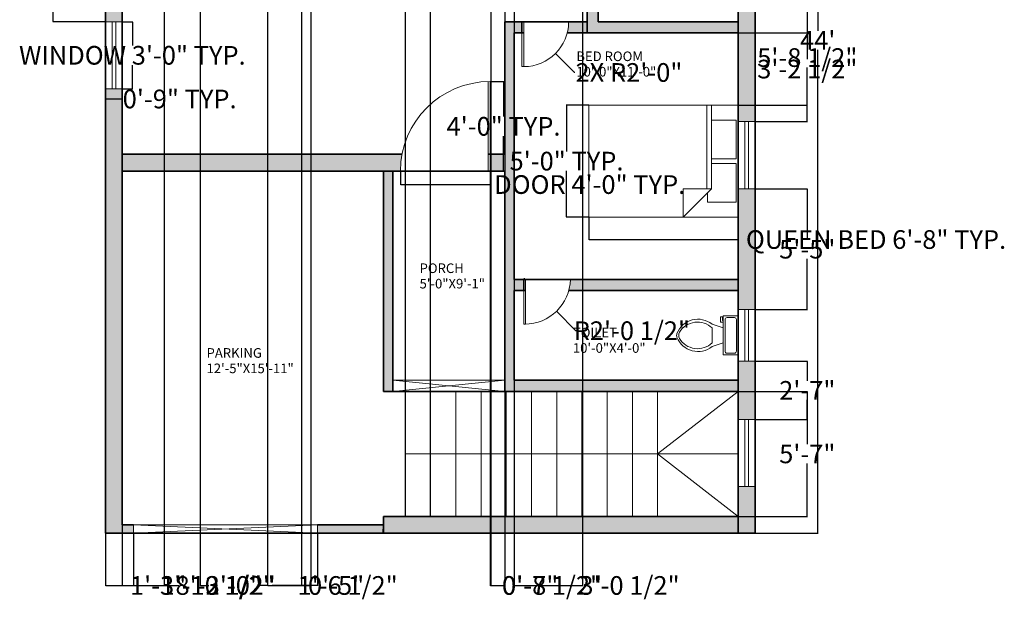
# Model space of a CAD drawing. Units: inches. Extents: x 2172 to 2712, y 1494 to 2108.
# Tile 1 of 3: x 2185 to 2712, y 1494 to 1812. Entities that reach past the tile are written whole.
import ezdxf

# ---------------------------------------------------------------- set-up
doc = ezdxf.new("R2010")
doc.units = ezdxf.units.IN
doc.header["$MEASUREMENT"] = 0
for name, color, linetype, lineweight in [('A-ANNO-DIMS', 2, 'Continuous', 18), ('A-AREA-IDEN', 7, 'Continuous', 18), ('A-DOOR', 3, 'Continuous', 18), ('A-FLOR-FIXT', 9, 'Continuous', 18), ('A-FLOR-STRS', 7, 'Continuous', 18), ('A-FURN', 8, 'Continuous', 18), ('A-GLAZ', 4, 'Continuous', 18), ('A-WALL', 7, 'Continuous', 35)]:
    doc.layers.add(name, color=color, linetype=linetype, lineweight=lineweight)
doc.layers.add('A-WALL-PATT', color=251, linetype='Continuous', lineweight=13, true_color=0x636466)
doc.styles.get("Standard").update_dxf_attribs({"font": 'arial.ttf'})
doc.dimstyles.get("Standard").update_dxf_attribs({"dimtxt": 10, "dimasz": 0.18, "dimexe": 0.18, "dimexo": 0.0625, "dimgap": 0.09, "dimtad": 0, "dimtih": 1, "dimtoh": 1, "dimdec": 0, "dimzin": 0, "dimdsep": 46, "dimlunit": 3, "dimtxsty": 'Standard', "dimcen": 0.09, "dimadec": 0, "dimazin": 0, "dimtfac": 1, "dimtdec": 0, "dimtofl": 0, "dimtmove": 0, "dimatfit": 3, "dimfxl": 1, "dimtolj": 1, "dimtzin": 0, "dimarcsym": 0})

# ---------------------------------------------------------------- blocks, each defined once
blk = doc.blocks.new('Toilet - top')
for p, q in [((9.5, -6), (9.5, -2)), ((-10, -8.5), (-8, -8.5)), ((-10, -9.5), (-10, -8.5)), ((-7, -9.5), (-10, -9.5)), ((-8, -8.5), (-8, -8)), ((-7, -8), (-7, -9.5)), ((-4, -8), (-6, -14)), ((4, -8), (6, -14)), ((4, -14), (-4, -14))]:
    blk.add_line(p, q)
blk.add_lwpolyline([(10.5, -8), (10.5, 0), (-10.5, 0), (-10.5, -8)], close=True)
for points in [[(-9.5, -2), (-9.5, -6)], [(8.5, -1), (-8.5, -1)], [(-8.5, -7), (8.5, -7)]]:
    blk.add_lwpolyline(points)
for centre, radius, start, end in [((-8.62, -1.88), 0.884, 81.8699, 188.1301), ((8.62, -1.88), 0.884, 351.8699, 98.1301), ((-8.62, -6.12), 0.884, 171.8699, 278.1301), ((8.62, -6.12), 0.884, 261.8699, 8.1301), ((3.52, -21.58), 12.17, 141.4691, 247.9714), ((4.2, -21.82), 11.33, 136.3677, 238.9468), ((-3.52, -21.58), 12.17, 292.0284, 38.5307), ((-4.2, -21.82), 11.33, 301.053, 43.6321), ((0, -27.88), 4, 245.7318, 294.2682), ((0, -29), 4, 254.8605, 285.1395)]:
    blk.add_arc(centre, radius, start, end)
blk = doc.blocks.new('Bed - Queen')
for p, q in [((0, -80.00003), (0, 0)), ((0, 0), (59.99999, 0)), ((59.99999, 0), (59.99999, -80.00003)), ((7.99999, -1.2), (28.79998, -1.2)), ((7.99999, -14.4), (7.99999, -1.2)), ((28.79998, -1.2), (28.79998, -14.4)), ((31.19999, -1.2), (51.99999, -1.2)), ((31.19999, -14.4), (31.19999, -1.2)), ((51.99999, -1.2), (51.99999, -16.4)), ((0, -14.4), (44.8, -14.4)), ((59.99999, -29.6), (44.8, -14.4)), ((44.8, -14.4), (44.8, -29.6)), ((44.8, -16.8), (0, -16.8)), ((51.99999, -16.4), (46.79936, -16.4)), ((44.8, -29.6), (59.99999, -29.6)), ((59.99999, -80.00003), (0, -80.00003))]:
    blk.add_line(p, q)
blk = doc.blocks.new('*D4')
at = {"layer": 'A-ANNO-DIMS', "color": 0, "lineweight": -2, "transparency": 16777216}
for p, q in [((2578.59, 2064.74), (2612.28, 2064.74)), ((2612.1, 2064.56), (2612.1, 1805.83)), ((2612.1, 1536.92), (2612.1, 1795.65)), ((2578.59, 1536.74), (2612.28, 1536.74))]:
    blk.add_line(p, q, dxfattribs=at)
at = {"layer": 'A-ANNO-DIMS', "color": 0, "transparency": 16777216}
for points in [[(2612.07, 2064.56), (2612.13, 2064.56), (2612.1, 2064.74)], [(2612.07, 1536.92), (2612.13, 1536.92), (2612.1, 1536.74)]]:
    blk.add_solid(points, dxfattribs=at)
at = {"layer": 'Defpoints', "color": 0, "transparency": 16777216}
for p in [(2578.53, 2064.74), (2578.53, 1536.74), (2612.1, 1536.74)]:
    blk.add_point(p, dxfattribs=at)
at = {"layer": 'A-ANNO-DIMS', "color": 0, "transparency": 16777216, "insert": (2612.1, 1800.74), "char_height": 10, "attachment_point": 5}
blk.add_mtext("\\A1;44'", dxfattribs=at)
blk = doc.blocks.new('WIN-36IN')
for p, q in [((0, 36), (9, 36)), ((3.5, 36), (3.5, 0)), ((5.5, 36), (5.5, 0)), ((9, 0), (0, 0))]:
    blk.add_line(p, q)
blk = doc.blocks.new('WIN-BATH-VENT')
for p, q in [((0, 27.69), (9, 27.69)), ((3.5, 27.69), (3.5, 0)), ((5.5, 27.69), (5.5, 0)), ((0, 0), (9, 0))]:
    blk.add_line(p, q)
blk = doc.blocks.new('DOOR-SWING-48IN')
for p, q in [((47, 0), (47, 48)), ((48, 0), (48, 48))]:
    blk.add_line(p, q)
blk.add_arc((48, 0), 48, 90, 180)
blk = doc.blocks.new('*D9')
at = {"layer": 'A-ANNO-DIMS', "color": 0, "lineweight": -2, "transparency": 16777216}
for p, q in [((2239.59, 1810.79), (2245.11, 1810.79)), ((2244.93, 1810.61), (2244.93, 1798.06)), ((2244.93, 1774.97), (2244.93, 1787.53)), ((2239.59, 1774.79), (2245.11, 1774.79))]:
    blk.add_line(p, q, dxfattribs=at)
at = {"layer": 'A-ANNO-DIMS', "color": 0, "transparency": 16777216}
for points in [[(2244.9, 1810.61), (2244.96, 1810.61), (2244.93, 1810.79)], [(2244.9, 1774.97), (2244.96, 1774.97), (2244.93, 1774.79)]]:
    blk.add_solid(points, dxfattribs=at)
at = {"layer": 'Defpoints', "color": 0, "transparency": 16777216}
for p in [(2239.53, 1810.79), (2244.93, 1810.79), (2239.53, 1774.79)]:
    blk.add_point(p, dxfattribs=at)
at = {"layer": 'A-ANNO-DIMS', "color": 0, "transparency": 16777216, "insert": (2244.93, 1792.79), "char_height": 10, "attachment_point": 5}
blk.add_mtext('\\A1;WINDOW 3\'-0" TYP.', dxfattribs=at)
blk = doc.blocks.new('*D10')
at = {"layer": 'A-ANNO-DIMS', "color": 0, "lineweight": -2, "transparency": 16777216}
for p, q in [((2230.53, 1774.73), (2230.53, 1769.21)), ((2239.53, 1774.73), (2239.53, 1769.21)), ((2230.71, 1769.39), (2239.35, 1769.39)), ((2239.53, 1769.39), (2239.71, 1769.39))]:
    blk.add_line(p, q, dxfattribs=at)
at = {"layer": 'A-ANNO-DIMS', "color": 0, "transparency": 16777216}
for points in [[(2230.71, 1769.42), (2230.71, 1769.36), (2230.53, 1769.39)], [(2239.35, 1769.42), (2239.35, 1769.36), (2239.53, 1769.39)]]:
    blk.add_solid(points, dxfattribs=at)
at = {"layer": 'Defpoints', "color": 0, "transparency": 16777216}
for p in [(2230.53, 1774.79), (2239.53, 1774.79), (2239.53, 1769.39)]:
    blk.add_point(p, dxfattribs=at)
at = {"layer": 'A-ANNO-DIMS', "color": 0, "transparency": 16777216, "insert": (2270.27, 1769.39), "char_height": 10, "attachment_point": 5}
blk.add_mtext('\\A1;0\'-9" TYP.', dxfattribs=at)
blk = doc.blocks.new('*D13')
at = {"layer": 'A-ANNO-DIMS', "color": 0, "lineweight": -2, "transparency": 16777216}
for p, q in [((2489.53, 1706.02), (2489.53, 1693.91)), ((2569.53, 1706.02), (2569.53, 1693.91)), ((2489.71, 1694.09), (2569.35, 1694.09)), ((2569.53, 1694.09), (2569.71, 1694.09))]:
    blk.add_line(p, q, dxfattribs=at)
at = {"layer": 'A-ANNO-DIMS', "color": 0, "transparency": 16777216}
for points in [[(2489.71, 1694.12), (2489.71, 1694.06), (2489.53, 1694.09)], [(2569.35, 1694.12), (2569.35, 1694.06), (2569.53, 1694.09)]]:
    blk.add_solid(points, dxfattribs=at)
at = {"layer": 'Defpoints', "color": 0, "transparency": 16777216}
for p in [(2489.53, 1706.09), (2569.53, 1706.09), (2569.53, 1694.09)]:
    blk.add_point(p, dxfattribs=at)
at = {"layer": 'A-ANNO-DIMS', "color": 0, "transparency": 16777216, "insert": (2643.35, 1694.09), "char_height": 10, "attachment_point": 5}
blk.add_mtext('\\A1;QUEEN BED 6\'-8" TYP.', dxfattribs=at)
blk = doc.blocks.new('*D14')
at = {"layer": 'A-ANNO-DIMS', "color": 0, "lineweight": -2, "transparency": 16777216}
for p, q in [((2489.46, 1766.09), (2477.35, 1766.09)), ((2477.53, 1765.91), (2477.53, 1741.28)), ((2477.53, 1706.27), (2477.53, 1730.89)), ((2489.46, 1706.09), (2477.35, 1706.09))]:
    blk.add_line(p, q, dxfattribs=at)
at = {"layer": 'A-ANNO-DIMS', "color": 0, "transparency": 16777216}
for points in [[(2477.5, 1765.91), (2477.56, 1765.91), (2477.53, 1766.09)], [(2477.5, 1706.27), (2477.56, 1706.27), (2477.53, 1706.09)]]:
    blk.add_solid(points, dxfattribs=at)
at = {"layer": 'Defpoints', "color": 0, "transparency": 16777216}
for p in [(2489.53, 1766.09), (2477.53, 1706.09), (2489.53, 1706.09)]:
    blk.add_point(p, dxfattribs=at)
at = {"layer": 'A-ANNO-DIMS', "color": 0, "transparency": 16777216, "insert": (2477.53, 1736.09), "char_height": 10, "attachment_point": 5}
blk.add_mtext('\\A1;5\'-0" TYP.', dxfattribs=at)
blk = doc.blocks.new('*D15')
at = {"layer": 'A-ANNO-DIMS', "color": 0, "lineweight": -2, "transparency": 16777216}
for p, q in [((2536.48, 1829.99), (2536.48, 1824.91)), ((2569.53, 1829.99), (2569.53, 1824.91)), ((2536.66, 1825.09), (2569.35, 1825.09)), ((2569.53, 1825.09), (2569.71, 1825.09))]:
    blk.add_line(p, q, dxfattribs=at)
at = {"layer": 'A-ANNO-DIMS', "color": 0, "transparency": 16777216}
for points in [[(2536.66, 1825.12), (2536.66, 1825.06), (2536.48, 1825.09)], [(2569.35, 1825.12), (2569.35, 1825.06), (2569.53, 1825.09)]]:
    blk.add_solid(points, dxfattribs=at)
at = {"layer": 'Defpoints', "color": 0, "transparency": 16777216}
for p in [(2536.48, 1830.05), (2569.53, 1830.05), (2569.53, 1825.09)]:
    blk.add_point(p, dxfattribs=at)
at = {"layer": 'A-ANNO-DIMS', "color": 0, "transparency": 16777216, "insert": (2614.06, 1825.09), "char_height": 10, "attachment_point": 5}
blk.add_mtext('\\A1;WC 2\'-9" TYP.', dxfattribs=at)
blk = doc.blocks.new('*D17')
at = {"layer": 'A-ANNO-DIMS', "color": 0, "lineweight": -2, "transparency": 16777216}
for p, q in [((2388.58, 1730.68), (2388.58, 1723.36)), ((2436.58, 1730.68), (2436.58, 1723.36)), ((2388.76, 1723.54), (2436.4, 1723.54)), ((2436.58, 1723.54), (2436.76, 1723.54))]:
    blk.add_line(p, q, dxfattribs=at)
at = {"layer": 'A-ANNO-DIMS', "color": 0, "transparency": 16777216}
for points in [[(2388.76, 1723.57), (2388.76, 1723.51), (2388.58, 1723.54)], [(2436.4, 1723.57), (2436.4, 1723.51), (2436.58, 1723.54)]]:
    blk.add_solid(points, dxfattribs=at)
at = {"layer": 'Defpoints', "color": 0, "transparency": 16777216}
for p in [(2388.58, 1730.74), (2436.58, 1730.74), (2436.58, 1723.54)]:
    blk.add_point(p, dxfattribs=at)
at = {"layer": 'A-ANNO-DIMS', "color": 0, "transparency": 16777216, "insert": (2489.97, 1723.54), "char_height": 10, "attachment_point": 5}
blk.add_mtext('\\A1;DOOR 4\'-0" TYP.', dxfattribs=at)
blk = doc.blocks.new('*D18')
at = {"layer": 'A-ANNO-DIMS', "color": 0, "lineweight": -2, "transparency": 16777216}
for p, q in [((2436.64, 1778.74), (2443.96, 1778.74)), ((2443.78, 1778.56), (2443.78, 1759.94)), ((2443.78, 1730.92), (2443.78, 1749.55)), ((2436.64, 1730.74), (2443.96, 1730.74))]:
    blk.add_line(p, q, dxfattribs=at)
at = {"layer": 'A-ANNO-DIMS', "color": 0, "transparency": 16777216}
for points in [[(2443.75, 1778.56), (2443.81, 1778.56), (2443.78, 1778.74)], [(2443.75, 1730.92), (2443.81, 1730.92), (2443.78, 1730.74)]]:
    blk.add_solid(points, dxfattribs=at)
at = {"layer": 'Defpoints', "color": 0, "transparency": 16777216}
for p in [(2436.58, 1778.74), (2443.78, 1778.74), (2436.58, 1730.74)]:
    blk.add_point(p, dxfattribs=at)
at = {"layer": 'A-ANNO-DIMS', "color": 0, "transparency": 16777216, "insert": (2443.78, 1754.74), "char_height": 10, "attachment_point": 5}
blk.add_mtext('\\A1;4\'-0" TYP.', dxfattribs=at)
blk = doc.blocks.new('*D23')
at = {"layer": 'A-ANNO-DIMS', "color": 0, "lineweight": -2, "transparency": 16777216}
for p, q in [((2230.46, 1884.82), (2202.35, 1884.82)), ((2202.53, 1884.64), (2202.53, 1853)), ((2202.53, 1810.97), (2202.53, 1842.61)), ((2230.46, 1810.79), (2202.35, 1810.79))]:
    blk.add_line(p, q, dxfattribs=at)
at = {"layer": 'A-ANNO-DIMS', "color": 0, "transparency": 16777216}
for points in [[(2202.5, 1884.64), (2202.56, 1884.64), (2202.53, 1884.82)], [(2202.5, 1810.97), (2202.56, 1810.97), (2202.53, 1810.79)]]:
    blk.add_solid(points, dxfattribs=at)
at = {"layer": 'Defpoints', "color": 0, "transparency": 16777216}
for p in [(2230.53, 1884.82), (2202.53, 1810.79), (2230.53, 1810.79)]:
    blk.add_point(p, dxfattribs=at)
at = {"layer": 'A-ANNO-DIMS', "color": 0, "transparency": 16777216, "insert": (2202.53, 1847.81), "char_height": 10, "attachment_point": 5}
blk.add_mtext('\\A1;6\'-2"', dxfattribs=at)
blk = doc.blocks.new('*D27')
at = {"layer": 'A-ANNO-DIMS', "color": 0, "lineweight": -2, "transparency": 16777216}
for p, q in [((2578.59, 1825.85), (2606.71, 1825.85)), ((2606.53, 1825.67), (2606.53, 1796.83)), ((2606.53, 1757.47), (2606.53, 1786.31)), ((2578.59, 1757.29), (2606.71, 1757.29))]:
    blk.add_line(p, q, dxfattribs=at)
at = {"layer": 'A-ANNO-DIMS', "color": 0, "transparency": 16777216}
for points in [[(2606.5, 1825.67), (2606.56, 1825.67), (2606.53, 1825.85)], [(2606.5, 1757.47), (2606.56, 1757.47), (2606.53, 1757.29)]]:
    blk.add_solid(points, dxfattribs=at)
at = {"layer": 'Defpoints', "color": 0, "transparency": 16777216}
for p in [(2578.53, 1825.85), (2578.53, 1757.29), (2606.53, 1757.29)]:
    blk.add_point(p, dxfattribs=at)
at = {"layer": 'A-ANNO-DIMS', "color": 0, "transparency": 16777216, "insert": (2606.53, 1791.57), "char_height": 10, "attachment_point": 5}
blk.add_mtext('\\A1;5\'-8 1/2"', dxfattribs=at)
blk = doc.blocks.new('*D28')
at = {"layer": 'A-ANNO-DIMS', "color": 0, "lineweight": -2, "transparency": 16777216}
for p, q in [((2578.59, 1721.29), (2606.71, 1721.29)), ((2606.53, 1721.11), (2606.53, 1694.08)), ((2606.53, 1656.71), (2606.53, 1683.73)), ((2578.59, 1656.53), (2606.71, 1656.53))]:
    blk.add_line(p, q, dxfattribs=at)
at = {"layer": 'A-ANNO-DIMS', "color": 0, "transparency": 16777216}
for points in [[(2606.5, 1721.11), (2606.56, 1721.11), (2606.53, 1721.29)], [(2606.5, 1656.71), (2606.56, 1656.71), (2606.53, 1656.53)]]:
    blk.add_solid(points, dxfattribs=at)
at = {"layer": 'Defpoints', "color": 0, "transparency": 16777216}
for p in [(2578.53, 1721.29), (2578.53, 1656.53), (2606.53, 1656.53)]:
    blk.add_point(p, dxfattribs=at)
at = {"layer": 'A-ANNO-DIMS', "color": 0, "transparency": 16777216, "insert": (2606.53, 1688.91), "char_height": 10, "attachment_point": 5}
blk.add_mtext('\\A1;5\'-5"', dxfattribs=at)
blk = doc.blocks.new('*D29')
at = {"layer": 'A-ANNO-DIMS', "color": 0, "lineweight": -2, "transparency": 16777216}
for p, q in [((2578.59, 1628.83), (2606.71, 1628.83)), ((2606.53, 1628.65), (2606.53, 1618.37)), ((2606.53, 1597.86), (2606.53, 1608.15)), ((2578.59, 1597.68), (2606.71, 1597.68))]:
    blk.add_line(p, q, dxfattribs=at)
at = {"layer": 'A-ANNO-DIMS', "color": 0, "transparency": 16777216}
for points in [[(2606.5, 1628.65), (2606.56, 1628.65), (2606.53, 1628.83)], [(2606.5, 1597.86), (2606.56, 1597.86), (2606.53, 1597.68)]]:
    blk.add_solid(points, dxfattribs=at)
at = {"layer": 'Defpoints', "color": 0, "transparency": 16777216}
for p in [(2578.53, 1628.83), (2578.53, 1597.68), (2606.53, 1597.68)]:
    blk.add_point(p, dxfattribs=at)
at = {"layer": 'A-ANNO-DIMS', "color": 0, "transparency": 16777216, "insert": (2606.53, 1613.26), "char_height": 10, "attachment_point": 5}
blk.add_mtext('\\A1;2\'-7"', dxfattribs=at)
blk = doc.blocks.new('*D30')
at = {"layer": 'A-ANNO-DIMS', "color": 0, "lineweight": -2, "transparency": 16777216}
for p, q in [((2230.53, 1536.68), (2230.53, 1508.56)), ((2245.63, 1536.68), (2245.63, 1508.56)), ((2230.71, 1508.74), (2245.45, 1508.74)), ((2245.63, 1508.74), (2245.81, 1508.74))]:
    blk.add_line(p, q, dxfattribs=at)
at = {"layer": 'A-ANNO-DIMS', "color": 0, "transparency": 16777216}
for points in [[(2230.71, 1508.77), (2230.71, 1508.71), (2230.53, 1508.74)], [(2245.45, 1508.77), (2245.45, 1508.71), (2245.63, 1508.74)]]:
    blk.add_solid(points, dxfattribs=at)
at = {"layer": 'Defpoints', "color": 0, "transparency": 16777216}
for p in [(2230.53, 1536.74), (2245.63, 1536.74), (2245.63, 1508.74)]:
    blk.add_point(p, dxfattribs=at)
at = {"layer": 'A-ANNO-DIMS', "color": 0, "transparency": 16777216, "insert": (2258.72, 1508.74), "char_height": 10, "attachment_point": 5}
blk.add_mtext('\\A1;1\'-3"', dxfattribs=at)
blk = doc.blocks.new('*D31')
at = {"layer": 'A-ANNO-DIMS', "color": 0, "lineweight": -2, "transparency": 16777216}
for p, q in [((2245.63, 1536.68), (2245.63, 1508.56)), ((2344.11, 1536.68), (2344.11, 1508.56)), ((2245.81, 1508.74), (2269.83, 1508.74)), ((2343.93, 1508.74), (2319.91, 1508.74))]:
    blk.add_line(p, q, dxfattribs=at)
at = {"layer": 'A-ANNO-DIMS', "color": 0, "transparency": 16777216}
for points in [[(2245.81, 1508.77), (2245.81, 1508.71), (2245.63, 1508.74)], [(2343.93, 1508.77), (2343.93, 1508.71), (2344.11, 1508.74)]]:
    blk.add_solid(points, dxfattribs=at)
at = {"layer": 'Defpoints', "color": 0, "transparency": 16777216}
for p in [(2245.63, 1536.74), (2344.11, 1536.74), (2344.11, 1508.74)]:
    blk.add_point(p, dxfattribs=at)
at = {"layer": 'A-ANNO-DIMS', "color": 0, "transparency": 16777216, "insert": (2294.87, 1508.74), "char_height": 10, "attachment_point": 5}
blk.add_mtext('\\A1;8\'-2 1/2"', dxfattribs=at)
blk = doc.blocks.new('*D32')
at = {"layer": 'A-ANNO-DIMS', "color": 0, "lineweight": -2, "transparency": 16777216}
for p, q in [((2391.23, 1545.8), (2391.23, 2092.92)), ((2391.41, 2092.74), (2404.56, 2092.74)), ((2404.74, 1545.8), (2404.74, 2092.92)), ((2404.74, 2092.74), (2404.92, 2092.74))]:
    blk.add_line(p, q, dxfattribs=at)
at = {"layer": 'A-ANNO-DIMS', "color": 0, "transparency": 16777216}
for points in [[(2391.41, 2092.77), (2391.41, 2092.71), (2391.23, 2092.74)], [(2404.56, 2092.77), (2404.56, 2092.71), (2404.74, 2092.74)]]:
    blk.add_solid(points, dxfattribs=at)
at = {"layer": 'Defpoints', "color": 0, "transparency": 16777216}
for p in [(2404.74, 2092.74), (2391.23, 1545.74), (2404.74, 1545.74)]:
    blk.add_point(p, dxfattribs=at)
at = {"layer": 'A-ANNO-DIMS', "color": 0, "transparency": 16777216, "insert": (2429.48, 2092.74), "char_height": 10, "attachment_point": 5}
blk.add_mtext('\\A1;1\'-1 1/2"', dxfattribs=at)
blk = doc.blocks.new('*D33')
at = {"layer": 'A-ANNO-DIMS', "color": 0, "lineweight": -2, "transparency": 16777216}
for p, q in [((2569.59, 1612.74), (2606.71, 1612.74)), ((2606.53, 1612.56), (2606.53, 1584.42)), ((2606.53, 1545.92), (2606.53, 1574.07)), ((2569.59, 1545.74), (2606.71, 1545.74))]:
    blk.add_line(p, q, dxfattribs=at)
at = {"layer": 'A-ANNO-DIMS', "color": 0, "transparency": 16777216}
for points in [[(2606.5, 1612.56), (2606.56, 1612.56), (2606.53, 1612.74)], [(2606.5, 1545.92), (2606.56, 1545.92), (2606.53, 1545.74)]]:
    blk.add_solid(points, dxfattribs=at)
at = {"layer": 'Defpoints', "color": 0, "transparency": 16777216}
for p in [(2569.53, 1612.74), (2606.53, 1612.74), (2569.53, 1545.74)]:
    blk.add_point(p, dxfattribs=at)
at = {"layer": 'A-ANNO-DIMS', "color": 0, "transparency": 16777216, "insert": (2606.53, 1579.24), "char_height": 10, "attachment_point": 5}
blk.add_mtext('\\A1;5\'-7"', dxfattribs=at)
blk = doc.blocks.new('*D34')
at = {"layer": 'A-ANNO-DIMS', "color": 0, "lineweight": -2, "transparency": 16777216}
for p, q in [((2239.53, 1935.68), (2239.53, 1508.56)), ((2261.99, 1935.68), (2261.99, 1508.56)), ((2239.71, 1508.74), (2261.81, 1508.74)), ((2261.99, 1508.74), (2262.17, 1508.74))]:
    blk.add_line(p, q, dxfattribs=at)
at = {"layer": 'A-ANNO-DIMS', "color": 0, "transparency": 16777216}
for points in [[(2239.71, 1508.77), (2239.71, 1508.71), (2239.53, 1508.74)], [(2261.81, 1508.77), (2261.81, 1508.71), (2261.99, 1508.74)]]:
    blk.add_solid(points, dxfattribs=at)
at = {"layer": 'Defpoints', "color": 0, "transparency": 16777216}
for p in [(2239.53, 1935.74), (2261.99, 1935.74), (2261.99, 1508.74)]:
    blk.add_point(p, dxfattribs=at)
at = {"layer": 'A-ANNO-DIMS', "color": 0, "transparency": 16777216, "insert": (2290.62, 1508.74), "char_height": 10, "attachment_point": 5}
blk.add_mtext('\\A1;1\'-10 1/2"', dxfattribs=at)
blk = doc.blocks.new('*D39')
at = {"layer": 'A-ANNO-DIMS', "color": 0, "lineweight": -2, "transparency": 16777216}
for p, q in [((2281.31, 2040.03), (2281.31, 1508.56)), ((2317.25, 2040.03), (2317.25, 1508.56)), ((2281.49, 1508.74), (2285.91, 1508.74)), ((2317.07, 1508.74), (2312.66, 1508.74))]:
    blk.add_line(p, q, dxfattribs=at)
at = {"layer": 'A-ANNO-DIMS', "color": 0, "transparency": 16777216}
for points in [[(2281.49, 1508.77), (2281.49, 1508.71), (2281.31, 1508.74)], [(2317.07, 1508.77), (2317.07, 1508.71), (2317.25, 1508.74)]]:
    blk.add_solid(points, dxfattribs=at)
at = {"layer": 'Defpoints', "color": 0, "transparency": 16777216}
for p in [(2281.31, 2040.1), (2317.25, 2040.1), (2317.25, 1508.74)]:
    blk.add_point(p, dxfattribs=at)
at = {"layer": 'A-ANNO-DIMS', "color": 0, "transparency": 16777216, "insert": (2299.28, 1508.74), "char_height": 10, "attachment_point": 5}
blk.add_mtext('\\A1;3\'-0"', dxfattribs=at)
blk = doc.blocks.new('*D41')
at = {"layer": 'A-ANNO-DIMS', "color": 0, "lineweight": -2, "transparency": 16777216}
for p, q in [((2437.05, 1929.68), (2437.05, 1508.56)), ((2444.53, 1929.68), (2444.53, 1508.56)), ((2437.23, 1508.74), (2444.35, 1508.74)), ((2444.53, 1508.74), (2444.71, 1508.74))]:
    blk.add_line(p, q, dxfattribs=at)
at = {"layer": 'A-ANNO-DIMS', "color": 0, "transparency": 16777216}
for points in [[(2437.23, 1508.77), (2437.23, 1508.71), (2437.05, 1508.74)], [(2444.35, 1508.77), (2444.35, 1508.71), (2444.53, 1508.74)]]:
    blk.add_solid(points, dxfattribs=at)
at = {"layer": 'Defpoints', "color": 0, "transparency": 16777216}
for p in [(2437.05, 1929.74), (2444.53, 1929.74), (2444.53, 1508.74)]:
    blk.add_point(p, dxfattribs=at)
at = {"layer": 'A-ANNO-DIMS', "color": 0, "transparency": 16777216, "insert": (2469.74, 1508.74), "char_height": 10, "attachment_point": 5}
blk.add_mtext('\\A1;0\'-7 1/2"', dxfattribs=at)
blk = doc.blocks.new('*D42')
at = {"layer": 'A-ANNO-DIMS', "color": 0, "lineweight": -2, "transparency": 16777216}
for p, q in [((2436.58, 1730.68), (2436.58, 1508.56)), ((2444.53, 1730.68), (2444.53, 1508.56)), ((2436.76, 1508.74), (2444.35, 1508.74)), ((2444.53, 1508.74), (2444.71, 1508.74))]:
    blk.add_line(p, q, dxfattribs=at)
at = {"layer": 'A-ANNO-DIMS', "color": 0, "transparency": 16777216}
for points in [[(2436.76, 1508.77), (2436.76, 1508.71), (2436.58, 1508.74)], [(2444.35, 1508.77), (2444.35, 1508.71), (2444.53, 1508.74)]]:
    blk.add_solid(points, dxfattribs=at)
at = {"layer": 'Defpoints', "color": 0, "transparency": 16777216}
for p in [(2436.58, 1730.74), (2444.53, 1730.74), (2444.53, 1508.74)]:
    blk.add_point(p, dxfattribs=at)
at = {"layer": 'A-ANNO-DIMS', "color": 0, "transparency": 16777216, "insert": (2458.09, 1508.74), "char_height": 10, "attachment_point": 5}
blk.add_mtext('\\A1;0\'-8"', dxfattribs=at)
blk = doc.blocks.new('*D43')
at = {"layer": 'A-ANNO-DIMS', "color": 0, "lineweight": -2, "transparency": 16777216}
for p, q in [((2335.53, 1941.85), (2335.53, 1508.56)), ((2340.53, 1941.85), (2340.53, 1508.56)), ((2335.71, 1508.74), (2340.35, 1508.74)), ((2340.53, 1508.74), (2340.71, 1508.74))]:
    blk.add_line(p, q, dxfattribs=at)
at = {"layer": 'A-ANNO-DIMS', "color": 0, "transparency": 16777216}
for points in [[(2335.71, 1508.77), (2335.71, 1508.71), (2335.53, 1508.74)], [(2340.35, 1508.77), (2340.35, 1508.71), (2340.53, 1508.74)]]:
    blk.add_solid(points, dxfattribs=at)
at = {"layer": 'Defpoints', "color": 0, "transparency": 16777216}
for p in [(2335.53, 1941.91), (2340.53, 1941.91), (2340.53, 1508.74)]:
    blk.add_point(p, dxfattribs=at)
at = {"layer": 'A-ANNO-DIMS', "color": 0, "transparency": 16777216, "insert": (2354.09, 1508.74), "char_height": 10, "attachment_point": 5}
blk.add_mtext('\\A1;0\'-5"', dxfattribs=at)
blk = doc.blocks.new('*D46')
at = {"layer": 'A-ANNO-DIMS', "color": 0, "lineweight": -2, "transparency": 16777216}
for p, q in [((2317.25, 2040.03), (2317.25, 1508.56)), ((2335.53, 2034.02), (2335.53, 1508.56)), ((2317.43, 1508.74), (2335.35, 1508.74)), ((2335.53, 1508.74), (2335.71, 1508.74))]:
    blk.add_line(p, q, dxfattribs=at)
at = {"layer": 'A-ANNO-DIMS', "color": 0, "transparency": 16777216}
for points in [[(2317.43, 1508.77), (2317.43, 1508.71), (2317.25, 1508.74)], [(2335.35, 1508.77), (2335.35, 1508.71), (2335.53, 1508.74)]]:
    blk.add_solid(points, dxfattribs=at)
at = {"layer": 'Defpoints', "color": 0, "transparency": 16777216}
for p in [(2317.25, 2040.1), (2335.53, 2034.09), (2335.53, 1508.74)]:
    blk.add_point(p, dxfattribs=at)
at = {"layer": 'A-ANNO-DIMS', "color": 0, "transparency": 16777216, "insert": (2360.27, 1508.74), "char_height": 10, "attachment_point": 5}
blk.add_mtext('\\A1;1\'-6 1/2"', dxfattribs=at)
blk = doc.blocks.new('*D47')
at = {"layer": 'A-ANNO-DIMS', "color": 0, "lineweight": -2, "transparency": 16777216}
for p, q in [((2449.53, 2055.68), (2449.53, 1508.56)), ((2486.06, 2055.68), (2486.06, 1508.56)), ((2449.71, 1508.74), (2485.88, 1508.74)), ((2486.06, 1508.74), (2486.24, 1508.74))]:
    blk.add_line(p, q, dxfattribs=at)
at = {"layer": 'A-ANNO-DIMS', "color": 0, "transparency": 16777216}
for points in [[(2449.71, 1508.77), (2449.71, 1508.71), (2449.53, 1508.74)], [(2485.88, 1508.77), (2485.88, 1508.71), (2486.06, 1508.74)]]:
    blk.add_solid(points, dxfattribs=at)
at = {"layer": 'Defpoints', "color": 0, "transparency": 16777216}
for p in [(2449.53, 2055.74), (2486.06, 2055.74), (2486.06, 1508.74)]:
    blk.add_point(p, dxfattribs=at)
at = {"layer": 'A-ANNO-DIMS', "color": 0, "transparency": 16777216, "insert": (2511.27, 1508.74), "char_height": 10, "attachment_point": 5}
blk.add_mtext('\\A1;3\'-0 1/2"', dxfattribs=at)
blk = doc.blocks.new('*D48')
at = {"layer": 'A-ANNO-DIMS', "color": 0, "lineweight": -2, "transparency": 16777216}
for p, q in [((2569.59, 1804.74), (2606.71, 1804.74)), ((2606.53, 1804.56), (2606.53, 1790.68)), ((2606.53, 1766.27), (2606.53, 1780.15)), ((2569.59, 1766.09), (2606.71, 1766.09))]:
    blk.add_line(p, q, dxfattribs=at)
at = {"layer": 'A-ANNO-DIMS', "color": 0, "transparency": 16777216}
for points in [[(2606.5, 1804.56), (2606.56, 1804.56), (2606.53, 1804.74)], [(2606.5, 1766.27), (2606.56, 1766.27), (2606.53, 1766.09)]]:
    blk.add_solid(points, dxfattribs=at)
at = {"layer": 'Defpoints', "color": 0, "transparency": 16777216}
for p in [(2569.53, 1804.74), (2569.53, 1766.09), (2606.53, 1766.09)]:
    blk.add_point(p, dxfattribs=at)
at = {"layer": 'A-ANNO-DIMS', "color": 0, "transparency": 16777216, "insert": (2606.53, 1785.41), "char_height": 10, "attachment_point": 5}
blk.add_mtext('\\A1;3\'-2 1/2"', dxfattribs=at)
blk = doc.blocks.new('*D49')
at = {"layer": 'A-ANNO-DIMS', "color": 0, "lineweight": -2, "transparency": 16777216}
for p, q in [((2455.01, 1673.25), (2455.19, 1673.25)), ((2455.1, 1673.16), (2455.1, 1673.34)), ((2482.53, 1645.24), (2472.37, 1655.61)), ((2482.71, 1645.24), (2482.53, 1645.24))]:
    blk.add_line(p, q, dxfattribs=at)
at = {"layer": 'A-ANNO-DIMS', "color": 0, "transparency": 16777216}
blk.add_solid([(2472.39, 1655.63), (2472.35, 1655.59), (2472.25, 1655.74)], dxfattribs=at)
at = {"layer": 'Defpoints', "color": 0, "transparency": 16777216}
for p in [(2455.1, 1673.25), (2472.25, 1655.74)]:
    blk.add_point(p, dxfattribs=at)
at = {"layer": 'A-ANNO-DIMS', "color": 0, "transparency": 16777216, "insert": (2512.53, 1645.24), "char_height": 10, "attachment_point": 5}
blk.add_mtext('\\A1;R2\'-0 1/2"', dxfattribs=at)
blk = doc.blocks.new('*D50')
at = {"layer": 'A-ANNO-DIMS', "color": 0, "lineweight": -2, "transparency": 16777216}
for p, q in [((2454.56, 1810.74), (2454.74, 1810.74)), ((2454.65, 1810.65), (2454.65, 1810.83)), ((2481.8, 1783.59), (2471.75, 1793.64)), ((2481.98, 1783.59), (2481.8, 1783.59))]:
    blk.add_line(p, q, dxfattribs=at)
at = {"layer": 'A-ANNO-DIMS', "color": 0, "transparency": 16777216}
blk.add_solid([(2471.77, 1793.66), (2471.72, 1793.62), (2471.62, 1793.77)], dxfattribs=at)
at = {"layer": 'Defpoints', "color": 0, "transparency": 16777216}
for p in [(2454.65, 1810.74), (2471.62, 1793.77)]:
    blk.add_point(p, dxfattribs=at)
at = {"layer": 'A-ANNO-DIMS', "color": 0, "transparency": 16777216, "insert": (2510.98, 1783.59), "char_height": 10, "attachment_point": 5}
blk.add_mtext('\\A1;2X R2\'-0"', dxfattribs=at)

msp = doc.modelspace()

# ---------------------------------------------------------------- hatches: boundary and pattern name
at = {"layer": 'A-WALL-PATT'}
h = msp.add_hatch(color=256, dxfattribs=at)
h.dxf.hatch_style = 1
h.paths.add_polyline_path([(2239.53, 1774.79), (2230.53, 1774.79), (2230.53, 1536.74), (2245.63, 1536.74), (2245.63, 1541.24), (2239.53, 1541.24)])
h.paths.add_polyline_path([(2569.53, 1545.74), (2379.53, 1545.74), (2379.53, 1536.74), (2569.53, 1536.74)])
h.paths.add_polyline_path([(2379.53, 1541.24), (2344.11, 1541.24), (2344.11, 1536.74), (2379.3, 1536.74)])
h.paths.add_polyline_path([(2578.53, 1561.68), (2569.53, 1561.68), (2569.53, 1536.74), (2578.53, 1536.74)])
h.paths.add_polyline_path([(2578.53, 1628.83), (2569.53, 1628.83), (2569.53, 1618.74), (2569.53, 1597.68), (2578.53, 1597.68)])
h.paths.add_polyline_path([(2578.53, 1721.29), (2569.53, 1721.29), (2569.53, 1672.74), (2569.53, 1656.53), (2578.53, 1656.53)])
h.paths.add_polyline_path([(2569.53, 1672.74), (2479.6, 1672.74, -0.062096), (2478.72, 1666.74), (2569.53, 1666.74)], flags=17)
h.paths.add_polyline_path([(2569.53, 1618.74), (2449.53, 1618.74), (2449.53, 1666.74), (2454.6, 1666.74), (2454.6, 1672.74), (2449.53, 1672.74), (2449.53, 1804.74), (2453.65, 1804.74), (2453.65, 1810.74), (2444.53, 1810.74), (2444.53, 1739.74), (2436.58, 1739.74), (2436.58, 1730.74), (2444.53, 1730.74), (2444.53, 1612.74), (2569.53, 1612.74)])
h.paths.add_polyline_path([(2384.53, 1730.74), (2379.53, 1730.74), (2379.53, 1612.74), (2384.53, 1612.74)])
h.paths.add_polyline_path([(2389.43, 1739.74), (2239.53, 1739.74), (2239.53, 1730.74), (2388.58, 1730.74, -0.047189)])
h.paths.add_polyline_path([(2569.53, 1810.74), (2494.53, 1810.74), (2494.53, 1832.1, -0.067617), (2488.53, 1831.74), (2488.53, 1830), (2488.53, 1804.74), (2569.53, 1804.74)])
h.paths.add_polyline_path([(2488.53, 1810.74), (2478.65, 1810.74, -0.063254), (2477.89, 1804.74), (2488.53, 1804.74)])
h.paths.add_polyline_path([(2569.53, 1864.74), (2488.53, 1864.74), (2488.53, 1858.74), (2569.53, 1858.74)])
h.paths.add_polyline_path([(2494.53, 1858.74), (2488.53, 1858.74), (2488.53, 1855), (2494.53, 1855)])
h.paths.add_polyline_path([(2494.53, 1887.05, -0.073561), (2488.53, 1888.74), (2488.53, 1885.18), (2488.53, 1879.18), (2488.53, 1864.74), (2494.53, 1864.74)])
h.paths.add_polyline_path([(2488.53, 1864.74), (2476.91, 1864.74, -0.063254), (2477.67, 1858.74), (2488.53, 1858.74)])
h.paths.add_polyline_path([(2449.53, 1918.74), (2449.53, 2055.74), (2444.53, 2055.74), (2444.53, 1912.74), (2444.53, 1858.74), (2449.53, 1858.74), (2452.67, 1858.74), (2452.67, 1864.74), (2449.53, 1864.74)])
h.paths.add_polyline_path([(2578.53, 1965.71), (2569.53, 1965.71), (2569.53, 1918.74), (2569.53, 1899.23), (2578.53, 1899.23)])
h.paths.add_polyline_path([(2578.53, 1825.85), (2569.53, 1825.85), (2569.53, 1757.29), (2578.53, 1757.29)])
h.paths.add_polyline_path([(2578.53, 1871.54), (2569.53, 1871.54), (2569.53, 1864.74), (2569.53, 1853.54), (2578.53, 1853.54)])
h.paths.add_polyline_path([(2239.53, 1884.82), (2230.53, 1884.82), (2230.53, 1810.79), (2239.53, 1810.79)])
h.paths.add_polyline_path([(2239.53, 1968.53), (2230.53, 1968.53), (2230.53, 1920.82), (2239.53, 1920.82), (2239.53, 1929.74)])
h.paths.add_polyline_path([(2389.42, 1935.74), (2340.53, 1935.74), (2340.53, 1941.91), (2335.53, 1941.91), (2335.53, 1935.74), (2239.53, 1935.74), (2239.53, 1929.74), (2340.53, 1929.74), (2389.05, 1929.74, -0.031342)])
h.paths.add_polyline_path([(2239.53, 2055.74), (2569.53, 2055.74), (2569.53, 2001.71), (2578.53, 2001.71), (2578.53, 2064.74), (2230.53, 2064.74), (2230.53, 2004.53), (2239.53, 2004.53)])
h.paths.add_polyline_path([(2340.53, 2055.74), (2335.53, 2055.74), (2335.53, 2008.15), (2340.53, 2008.15)], flags=17)
h.paths.add_polyline_path([(2444.53, 1935.74), (2437.05, 1935.74), (2437.05, 1929.74), (2444.53, 1929.74)])
h.paths.add_polyline_path([(2569.53, 1918.74), (2488.53, 1918.74), (2488.53, 1909.18), (2494.53, 1909.18), (2494.53, 1912.74), (2569.53, 1912.74)])

# ---------------------------------------------------------------- linework, layer by layer
at = {"layer": 'A-DOOR'}
for p, q in [((2453.65, 1810.74), (2453.65, 1786.74)), ((2454.65, 1786.74), (2454.65, 1810.74)), ((2454.65, 1810.74), (2454.65, 1810.74)), ((2454.65, 1810.74), (2478.65, 1810.74)), ((2453.65, 1786.74), (2454.65, 1786.74)), ((2454.6, 1672.74), (2454.6, 1648.74)), ((2455.6, 1648.74), (2455.6, 1672.74)), ((2455.6, 1672.74), (2479.6, 1672.74)), ((2454.6, 1648.74), (2455.6, 1648.74)), ((2444.53, 1618.74), (2384.53, 1618.74)), ((2384.53, 1612.74), (2444.53, 1618.74)), ((2384.53, 1618.74), (2444.53, 1612.74)), ((2245.63, 1541.24), (2245.63, 1536.74)), ((2245.63, 1536.74), (2344.11, 1541.24)), ((2344.11, 1536.74), (2245.63, 1541.24)), ((2245.63, 1541.24), (2344.11, 1541.24)), ((2344.11, 1541.24), (2344.11, 1536.74)), ((2344.11, 1536.74), (2344.11, 1541.24))]:
    msp.add_line(p, q, dxfattribs=at)
for centre, radius, end in [((2454.65, 1810.74), 24, 0), ((2455.1, 1673.25), 24.51, 358.8187)]:
    msp.add_arc(centre, radius, 270, end, dxfattribs=at)
at = {"layer": 'A-FLOR-STRS'}
for p, q in [((2391.23, 1545.74), (2391.23, 1612.74)), ((2404.74, 1545.74), (2404.74, 1612.74)), ((2418.25, 1545.74), (2418.25, 1612.74)), ((2431.76, 1545.74), (2431.76, 1612.74)), ((2445.27, 1545.74), (2445.27, 1612.74)), ((2458.78, 1545.74), (2458.78, 1612.74)), ((2472.29, 1545.74), (2472.29, 1612.74)), ((2485.8, 1545.74), (2485.8, 1612.74)), ((2499.31, 1545.74), (2499.31, 1612.74)), ((2512.82, 1545.74), (2512.82, 1612.74)), ((2526.33, 1545.74), (2526.33, 1612.74)), ((2526.33, 1579.24), (2569.53, 1612.74)), ((2517.85, 1579.24), (2391.23, 1579.24)), ((2391.23, 1579.24), (2569.53, 1579.24)), ((2526.33, 1579.24), (2517.85, 1579.24)), ((2526.33, 1579.24), (2569.53, 1545.74))]:
    msp.add_line(p, q, dxfattribs=at)
at = {"layer": 'A-GLAZ'}
msp.add_line((2574.03, 1628.83), (2569.53, 1628.83), dxfattribs=at)
at = {"layer": 'A-WALL'}
for p, q in [((2230.53, 2064.74), (2230.53, 1536.74)), ((2578.53, 2064.74), (2578.53, 1536.74)), ((2239.53, 2055.74), (2239.53, 1541.24)), ((2569.53, 2055.74), (2569.53, 1536.74)), ((2239.53, 1929.74), (2239.53, 1739.74)), ((2488.53, 1804.74), (2488.53, 1858.74)), ((2569.53, 1858.74), (2569.53, 1810.74)), ((2494.53, 1810.74), (2494.53, 1832.1)), ((2444.53, 1810.74), (2488.53, 1810.74)), ((2444.53, 1739.74), (2444.53, 1810.74)), ((2453.65, 1804.74), (2453.65, 1810.74)), ((2569.53, 1810.74), (2494.53, 1810.74)), ((2449.53, 1672.74), (2449.53, 1804.74)), ((2449.53, 1804.74), (2454.65, 1804.74)), ((2477.89, 1804.74), (2488.53, 1804.74)), ((2569.53, 1804.74), (2488.53, 1804.74)), ((2569.53, 1804.74), (2569.53, 1672.74)), ((2239.53, 1739.74), (2389.43, 1739.74)), ((2435.58, 1739.74), (2444.53, 1739.74)), ((2239.53, 1730.74), (2444.53, 1730.74)), ((2379.53, 1612.74), (2379.53, 1730.74)), ((2384.53, 1612.74), (2384.53, 1730.74)), ((2444.53, 1730.74), (2444.53, 1666.74)), ((2444.53, 1730.74), (2444.53, 1612.74)), ((2569.53, 1672.74), (2449.53, 1672.74)), ((2454.6, 1672.74), (2454.6, 1666.74)), ((2444.53, 1666.74), (2444.53, 1618.74)), ((2449.53, 1618.74), (2449.53, 1666.74)), ((2455.6, 1666.74), (2449.53, 1666.74)), ((2569.53, 1666.74), (2478.72, 1666.74)), ((2569.53, 1666.74), (2569.53, 1618.74)), ((2569.53, 1618.74), (2449.53, 1618.74)), ((2444.53, 1612.74), (2379.53, 1612.74)), ((2569.53, 1612.74), (2444.53, 1612.74)), ((2379.53, 1545.74), (2569.53, 1545.74)), ((2379.53, 1545.74), (2379.53, 1536.74)), ((2245.63, 1541.24), (2239.53, 1541.24)), ((2379.53, 1541.24), (2344.11, 1541.24)), ((2379.3, 1536.74), (2379.53, 1541.24)), ((2230.53, 1536.74), (2578.53, 1536.74)), ((2569.53, 1536.74), (2379.3, 1536.74)), ((2379.53, 1536.74), (2569.53, 1536.74))]:
    msp.add_line(p, q, dxfattribs=at)

# ---------------------------------------------------------------- block references
at = {"layer": 'A-DOOR'}
msp.add_blockref('DOOR-SWING-48IN', (2388.58, 1730.74), dxfattribs=at)
at = {"layer": 'A-FLOR-FIXT', "rotation": 270}
msp.add_blockref('Toilet - top', (2569.53, 1642.74), dxfattribs=at)
at = {"layer": 'A-FURN', "rotation": 270}
msp.add_blockref('Bed - Queen', (2569.53, 1766.09), dxfattribs=at)
at = {"layer": 'A-GLAZ'}
for name, p in [('WIN-36IN', (2230.53, 1774.79)), ('WIN-36IN', (2569.53, 1721.29)), ('WIN-BATH-VENT', (2569.53, 1628.84)), ('WIN-36IN', (2569.53, 1561.68))]:
    msp.add_blockref(name, p, dxfattribs=at)

# ---------------------------------------------------------------- texts
at = {"layer": 'A-AREA-IDEN'}
for s, height, p in [('BED ROOM', 5.144, (2482.79, 1789.69)), ('10\'-0"X11\'-0"', 5.1443, (2482.79, 1781.42)), ('PORCH', 5.144, (2398.8, 1676.14)), ('5\'-0"X9\'-1"', 5.1443, (2398.8, 1667.88)), ('TOILET', 5.144, (2480.94, 1641.67)), ('PARKING ', 5.144, (2284.67, 1630.75)), ('10\'-0"X4\'-0"', 5.1443, (2480.94, 1633.4)), ('12\'-5"X15\'-11"', 5.1443, (2284.67, 1622.49))]:
    msp.add_text(s, height=height, dxfattribs=at).set_placement(p)

# ---------------------------------------------------------------- dimensions: what is measured, and where the dimension line sits
at = {"layer": 'A-ANNO-DIMS'}
for base, p1, p2, picture, middle in [((2404.74, 2092.74), (2391.23, 1545.74), (2404.74, 1545.74), '*D32', (2429.48, 2092.74)), ((2486.06, 1508.74), (2449.53, 2055.74), (2486.06, 2055.74), '*D47', (2511.27, 1508.74)), ((2317.25, 1508.74), (2281.31, 2040.1), (2317.25, 2040.1), '*D39', (2299.28, 1508.74)), ((2335.53, 1508.74), (2317.25, 2040.1), (2335.53, 2034.09), '*D46', (2360.27, 1508.74)), ((2340.53, 1508.74), (2335.53, 1941.91), (2340.53, 1941.91), '*D43', (2354.09, 1508.74)), ((2261.99, 1508.74), (2239.53, 1935.74), (2261.99, 1935.74), '*D34', (2290.62, 1508.74)), ((2444.53, 1508.74), (2437.05, 1929.74), (2444.53, 1929.74), '*D41', (2469.74, 1508.74)), ((2444.5253, 1508.7407), (2436.5767, 1730.7407), (2444.5253, 1730.7407), '*D42', (2458.0865, 1508.7407)), ((2245.63, 1508.74), (2230.53, 1536.74), (2245.63, 1536.74), '*D30', (2258.72, 1508.74)), ((2344.11, 1508.74), (2245.63, 1536.74), (2344.11, 1536.74), '*D31', (2294.87, 1508.74))]:
    dim = msp.add_linear_dim(base=base, p1=p1, p2=p2, dimstyle='Standard', override={"dimdec": 1, "dimlfac": 1, "dimrnd": 0, "dimzin": 1, "dimdsep": 46, "dimlunit": 4, "dimfrac": 2}, dxfattribs=at)
    dim.commit()
    dim.dimension.update_dxf_attribs({"geometry": picture, "text_midpoint": middle})
for base, p1, p2, override, picture, middle in [((2612.1, 1536.74), (2578.53, 2064.74), (2578.53, 1536.74), {"dimclrd": 0, "dimclre": 0, "dimclrt": 0}, '*D4', (2612.1, 1800.74)), ((2202.53, 1810.79), (2230.53, 1884.82), (2230.53, 1810.79), {"dimdec": 1, "dimlfac": 1, "dimrnd": 0, "dimzin": 1, "dimdsep": 46, "dimlunit": 4, "dimfrac": 2}, '*D23', (2202.53, 1847.81)), ((2606.53, 1757.29), (2578.53, 1825.85), (2578.53, 1757.29), {"dimdec": 1, "dimlfac": 1, "dimrnd": 0, "dimzin": 1, "dimdsep": 46, "dimlunit": 4, "dimfrac": 2}, '*D27', (2606.53, 1791.57)), ((2606.5253, 1766.0861), (2569.5253, 1804.7407), (2569.5253, 1766.0861), {"dimdec": 1, "dimlfac": 1, "dimrnd": 0, "dimzin": 1, "dimdsep": 46, "dimlunit": 4, "dimfrac": 2}, '*D48', (2606.5253, 1785.4134)), ((2606.53, 1656.53), (2578.53, 1721.29), (2578.53, 1656.53), {"dimdec": 1, "dimlfac": 1, "dimrnd": 0, "dimzin": 1, "dimdsep": 46, "dimlunit": 4, "dimfrac": 2}, '*D28', (2606.53, 1688.91)), ((2606.5253, 1597.6783), (2578.5253, 1628.8347), (2578.5253, 1597.6783), {"dimdec": 1, "dimlfac": 1, "dimrnd": 0, "dimzin": 1, "dimdsep": 46, "dimlunit": 4, "dimfrac": 2}, '*D29', (2606.5253, 1613.2565)), ((2606.53, 1612.74), (2569.53, 1545.74), (2569.53, 1612.74), {"dimdec": 1, "dimlfac": 1, "dimrnd": 0, "dimzin": 1, "dimdsep": 46, "dimlunit": 4, "dimfrac": 2}, '*D33', (2606.53, 1579.24))]:
    dim = msp.add_linear_dim(base=base, p1=p1, p2=p2, angle=90, dimstyle='Standard', override=override, dxfattribs=at)
    dim.commit()
    dim.dimension.update_dxf_attribs({"geometry": picture, "text_midpoint": middle})
for base, p1, p2, text, picture, middle in [((2569.5253, 1825.0942), (2536.479, 1830.0512), (2569.5253, 1830.0512), 'WC <> TYP.', '*D15', (2614.0552, 1825.0942)), ((2239.53, 1769.39), (2230.53, 1774.79), (2239.53, 1774.79), '<> TYP.', '*D10', (2270.27, 1769.39)), ((2436.58, 1723.54), (2388.58, 1730.74), (2436.58, 1730.74), 'DOOR <> TYP.', '*D17', (2489.97, 1723.54)), ((2569.53, 1694.09), (2489.53, 1706.09), (2569.53, 1706.09), 'QUEEN BED <> TYP.', '*D13', (2643.35, 1694.09))]:
    dim = msp.add_linear_dim(base=base, p1=p1, p2=p2, text=text, dimstyle='Standard', override={"dimdec": 1, "dimlfac": 1, "dimrnd": 0, "dimzin": 1, "dimdsep": 46, "dimlunit": 4, "dimfrac": 2}, dxfattribs=at)
    dim.commit()
    dim.dimension.update_dxf_attribs({"geometry": picture, "text_midpoint": middle})
for base, p1, p2, angle, text, picture, middle in [((2244.93, 1810.79), (2239.53, 1774.79), (2239.53, 1810.79), 90, 'WINDOW <> TYP.', '*D9', (2244.93, 1792.79)), ((2443.78, 1778.74), (2436.58, 1730.74), (2436.58, 1778.74), 90, '<> TYP.', '*D18', (2443.78, 1754.74)), ((2477.53, 1706.09), (2489.53, 1766.09), (2489.53, 1706.09), 270, '<> TYP.', '*D14', (2477.53, 1736.09))]:
    dim = msp.add_linear_dim(base=base, p1=p1, p2=p2, angle=angle, text=text, dimstyle='Standard', override={"dimdec": 1, "dimlfac": 1, "dimrnd": 0, "dimzin": 1, "dimdsep": 46, "dimlunit": 4, "dimfrac": 2}, dxfattribs=at)
    dim.commit()
    dim.dimension.update_dxf_attribs({"geometry": picture, "text_midpoint": middle})
dim = msp.add_radius_dim(center=(2454.65, 1810.74), mpoint=(2471.62, 1793.77), text='2X <>', dimstyle='Standard', override={"dimdec": 1, "dimlfac": 1, "dimrnd": 0, "dimzin": 1, "dimdsep": 46, "dimlunit": 4, "dimfrac": 2}, dxfattribs=at)
dim.commit()
dim.dimension.update_dxf_attribs({"geometry": '*D50', "text_midpoint": (2510.98, 1783.59), "dimtype": 164})
dim = msp.add_radius_dim(center=(2455.1, 1673.25), mpoint=(2472.25, 1655.74), dimstyle='Standard', override={"dimdec": 1, "dimlfac": 1, "dimrnd": 0, "dimzin": 1, "dimdsep": 46, "dimlunit": 4, "dimfrac": 2}, dxfattribs=at)
dim.commit()
dim.dimension.update_dxf_attribs({"geometry": '*D49', "text_midpoint": (2512.53, 1645.24), "dimtype": 164})

doc.saveas('drawing.dxf')
